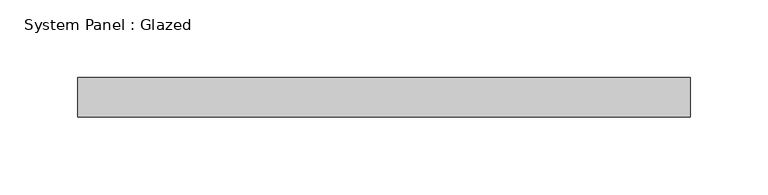
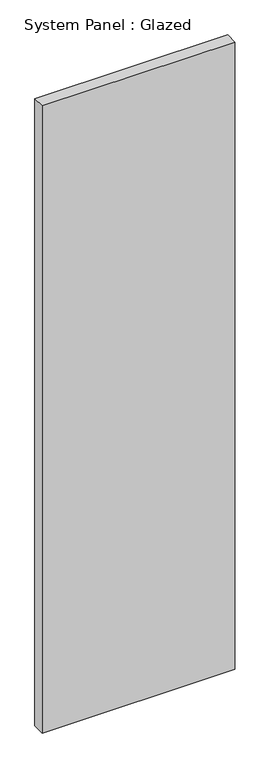
"""IFC4 building model written with IfcOpenShell, lengths in millimetres: plate geometry, System Panel : Glazed."""

from ifc_helpers import new_model, si_unit, origin, origin_with_axes, place, context, project, spatial, polyline, outline, extrude, source, transform, mapped, element, save


def system_panel_glazed_ba1f660c(model_context):
    return source(origin(), model_context, "Body", "SweptSolid", [
        extrude(outline(polyline([(196.85, -44.45), (-196.85, -44.45), (-196.85, -19.05), (196.85, -19.05), (196.85, -44.45)])), origin_with_axes(), (0.0, 0.0, 1.0), 1355.4314829),
    ])


if __name__ == "__main__":
    model = new_model("IFC4")
    model_context = context("Model", 3, world=origin())
    ifc_project = project(units=[si_unit("LENGTHUNIT", "METRE", prefix="MILLI")], contexts=[model_context])
    site = spatial("IfcSite", under=ifc_project)
    building = spatial("IfcBuilding", under=site)
    placement = place(None, origin())
    system_panel_glazed_shape = system_panel_glazed_ba1f660c(model_context)
    element("IfcPlate", 1, ObjectType="System Panel : Glazed", at=placement, inside=building, context=model_context, shape_type="MappedRepresentation", body=[
        mapped(system_panel_glazed_shape, transform((0.0, 0.0, 0.0), x_axis=(1.0, 0.0, 0.0), y_axis=(0.0, 1.0, 0.0), z_axis=(0.0, 0.0, 1.0))),
    ])
    save(model, "model.ifc")

# Revit data of these elements
# Type "System Panel : Glazed"
#   Construction Type Id = "GSP4R"
#   Analytic Construction = "1/8 in Pilkington single glazing"
#   Visual Light Transmittance = 0.9
#   Solar Heat Gain Coefficient = 0.86
#   Heat Transfer Coefficient (U) = 1.18115 BTU/(h·ft²·°F)
#   Define Thermal Properties by = 1
# Element 1 (IfcPlate, "System Panel : Glazed")
#   Materials on its faces: "Glass"
# Materials
#   "Glass": class "Glass", colour RGB 0 128 192, transparency 0.75, Description = "Soda Lime Glass", Cost = 0
